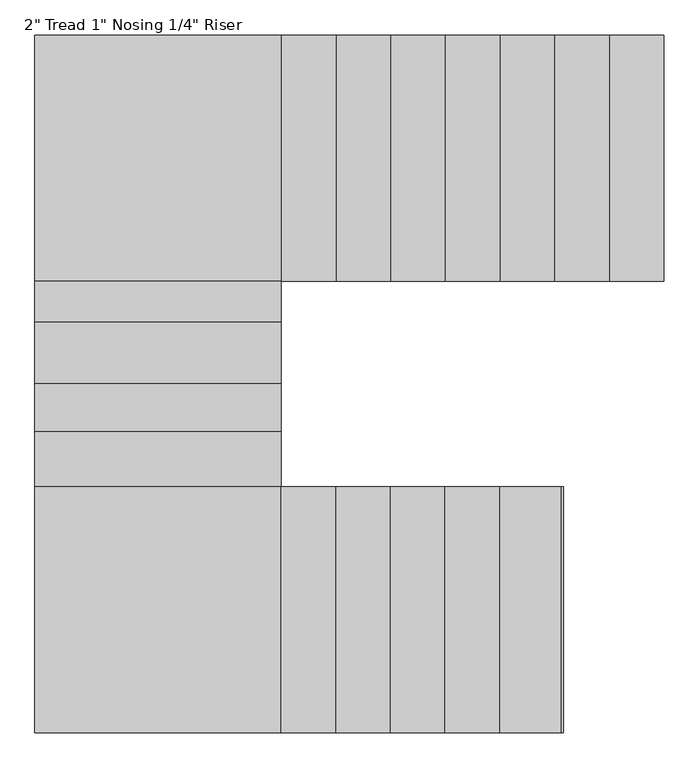
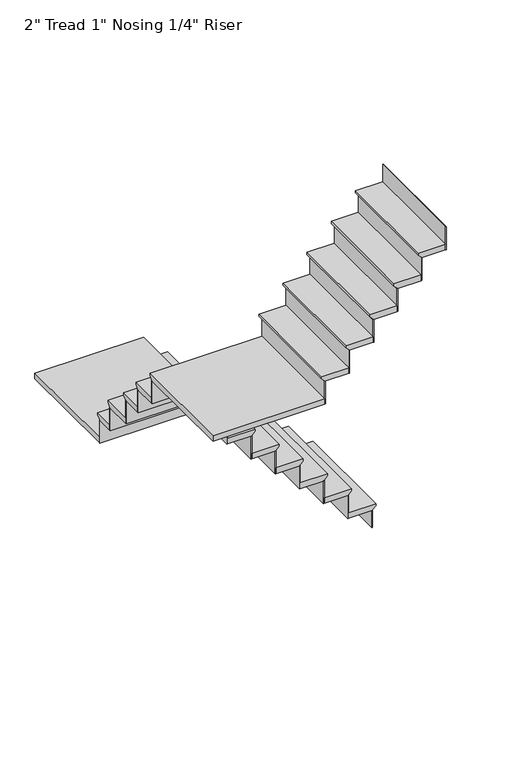
"""IFC4 building model written with IfcOpenShell, lengths in millimetres: stair flight geometry."""

from ifc_helpers import new_model, si_unit, origin, place, context, project, spatial, faceted_brep, source, transform, mapped, element, save


def stair_flight_8f890541(model_context):
    return source(origin(), model_context, "Body", "Brep", [
        faceted_brep([(-3603.1340247, 922.0319954, 184.15), (-3603.1340247, 922.0319954, 203.2), (-3603.1340247, 7.6319954, 203.2), (-3603.1340247, 7.6319954, 184.15), (-3628.5340247, 922.0319954, 158.75), (-3628.5340247, 7.6319954, 158.75), (-3831.7340247, 922.0319954, 203.2), (-3831.7340247, 7.6319954, 203.2), (-3628.5340247, 7.6319954, 152.4), (-3831.7340247, 7.6319954, 152.4), (-3831.7340247, 922.0319954, 152.4), (-3628.5340247, 922.0319954, 152.4)], [[[0, 1, 2, 3]], [[4, 0, 3, 5]], [[2, 1, 6, 7]], [[8, 9, 10, 11]], [[2, 7, 9, 8, 5, 3]], [[8, 11, 4, 5]], [[6, 1, 0, 4, 11, 10]], [[7, 6, 10, 9]]]),
        faceted_brep([(-3628.5340247, 922.0319954, 152.4), (-3628.5340247, 922.0319954, 0.0), (-3634.8840247, 922.0319954, 0.0), (-3634.8840247, 922.0319954, 152.4), (-3628.5340247, 7.6319954, 152.4), (-3634.8840247, 7.6319954, 152.4), (-3634.8840247, 7.6319954, 0.0), (-3628.5340247, 7.6319954, 0.0)], [[[0, 1, 2, 3]], [[4, 5, 6, 7]], [[1, 0, 4, 7]], [[2, 1, 7, 6]], [[3, 2, 6, 5]], [[0, 3, 5, 4]]]),
        faceted_brep([(-3831.7340247, 922.0319954, 355.6), (-3831.7340247, 922.0319954, 152.4), (-3838.0840247, 922.0319954, 152.4), (-3838.0840247, 922.0319954, 355.6), (-3831.7340247, 7.6319954, 355.6), (-3838.0840247, 7.6319954, 355.6), (-3838.0840247, 7.6319954, 152.4), (-3831.7340247, 7.6319954, 152.4)], [[[0, 1, 2, 3]], [[4, 5, 6, 7]], [[1, 0, 4, 7]], [[2, 1, 7, 6]], [[3, 2, 6, 5]], [[0, 3, 5, 4]]]),
        faceted_brep([(-3806.3340247, 7.6319954, 406.4), (-3806.3340247, 922.0319954, 406.4), (-4034.9340247, 922.0319954, 406.4), (-4034.9340247, 7.6319954, 406.4), (-3831.7340247, 7.6319954, 355.6), (-4034.9340247, 7.6319954, 355.6), (-4034.9340247, 922.0319954, 355.6), (-3831.7340247, 922.0319954, 355.6), (-3831.7340247, 7.6319954, 361.95), (-3806.3340247, 7.6319954, 387.35), (-3831.7340247, 922.0319954, 361.95), (-3806.3340247, 922.0319954, 387.35)], [[[0, 1, 2, 3]], [[4, 5, 6, 7]], [[0, 3, 5, 4, 8, 9]], [[4, 7, 10, 8]], [[2, 1, 11, 10, 7, 6]], [[3, 2, 6, 5]], [[11, 1, 0, 9]], [[10, 11, 9, 8]]]),
        faceted_brep([(-4034.9340247, 922.0319954, 558.8), (-4034.9340247, 922.0319954, 355.6), (-4041.2840247, 922.0319954, 355.6), (-4041.2840247, 922.0319954, 558.8), (-4034.9340247, 7.6319954, 558.8), (-4041.2840247, 7.6319954, 558.8), (-4041.2840247, 7.6319954, 355.6), (-4034.9340247, 7.6319954, 355.6)], [[[0, 1, 2, 3]], [[4, 5, 6, 7]], [[1, 0, 4, 7]], [[2, 1, 7, 6]], [[3, 2, 6, 5]], [[0, 3, 5, 4]]]),
        faceted_brep([(-4009.5340247, 7.6319954, 609.6), (-4009.5340247, 922.0319954, 609.6), (-4238.1340247, 922.0319954, 609.6), (-4238.1340247, 7.6319954, 609.6), (-4034.9340247, 7.6319954, 558.8), (-4238.1340247, 7.6319954, 558.8), (-4238.1340247, 922.0319954, 558.8), (-4034.9340247, 922.0319954, 558.8), (-4034.9340247, 7.6319954, 565.15), (-4009.5340247, 7.6319954, 590.55), (-4034.9340247, 922.0319954, 565.15), (-4009.5340247, 922.0319954, 590.55)], [[[0, 1, 2, 3]], [[4, 5, 6, 7]], [[0, 3, 5, 4, 8, 9]], [[4, 7, 10, 8]], [[2, 1, 11, 10, 7, 6]], [[3, 2, 6, 5]], [[11, 1, 0, 9]], [[10, 11, 9, 8]]]),
        faceted_brep([(-4238.1340247, 922.0319954, 762.0), (-4238.1340247, 922.0319954, 558.8), (-4244.4840247, 922.0319954, 558.8), (-4244.4840247, 922.0319954, 762.0), (-4238.1340247, 7.6319954, 762.0), (-4244.4840247, 7.6319954, 762.0), (-4244.4840247, 7.6319954, 558.8), (-4238.1340247, 7.6319954, 558.8)], [[[0, 1, 2, 3]], [[4, 5, 6, 7]], [[1, 0, 4, 7]], [[2, 1, 7, 6]], [[3, 2, 6, 5]], [[0, 3, 5, 4]]]),
        faceted_brep([(-4212.7340247, 7.6319954, 812.8), (-4212.7340247, 922.0319954, 812.8), (-4441.3340247, 922.0319954, 812.8), (-4441.3340247, 7.6319954, 812.8), (-4238.1340247, 7.6319954, 762.0), (-4441.3340247, 7.6319954, 762.0), (-4441.3340247, 922.0319954, 762.0), (-4238.1340247, 922.0319954, 762.0), (-4238.1340247, 7.6319954, 768.35), (-4212.7340247, 7.6319954, 793.75), (-4238.1340247, 922.0319954, 768.35), (-4212.7340247, 922.0319954, 793.75)], [[[0, 1, 2, 3]], [[4, 5, 6, 7]], [[0, 3, 5, 4, 8, 9]], [[4, 7, 10, 8]], [[2, 1, 11, 10, 7, 6]], [[3, 2, 6, 5]], [[11, 1, 0, 9]], [[10, 11, 9, 8]]]),
        faceted_brep([(-4441.3340247, 922.0319954, 965.2), (-4441.3340247, 922.0319954, 762.0), (-4447.6840247, 922.0319954, 762.0), (-4447.6840247, 922.0319954, 965.2), (-4441.3340247, 7.6319954, 965.2), (-4447.6840247, 7.6319954, 965.2), (-4447.6840247, 7.6319954, 762.0), (-4441.3340247, 7.6319954, 762.0)], [[[0, 1, 2, 3]], [[4, 5, 6, 7]], [[1, 0, 4, 7]], [[2, 1, 7, 6]], [[3, 2, 6, 5]], [[0, 3, 5, 4]]]),
        faceted_brep([(-4415.9340247, 7.6319954, 1016.0), (-4415.9340247, 922.0319954, 1016.0), (-4644.5340247, 922.0319954, 1016.0), (-4644.5340247, 7.6319954, 1016.0), (-4441.3340247, 7.6319954, 965.2), (-4644.5340247, 7.6319954, 965.2), (-4644.5340247, 922.0319954, 965.2), (-4441.3340247, 922.0319954, 965.2), (-4441.3340247, 7.6319954, 971.55), (-4415.9340247, 7.6319954, 996.95), (-4441.3340247, 922.0319954, 971.55), (-4415.9340247, 922.0319954, 996.95)], [[[0, 1, 2, 3]], [[4, 5, 6, 7]], [[0, 3, 5, 4, 8, 9]], [[4, 7, 10, 8]], [[2, 1, 11, 10, 7, 6]], [[3, 2, 6, 5]], [[11, 1, 0, 9]], [[10, 11, 9, 8]]]),
        faceted_brep([(-4644.5340247, 922.0319954, 1168.4), (-4644.5340247, 922.0319954, 965.2), (-4650.8840247, 922.0319954, 965.2), (-4650.8840247, 922.0319954, 1168.4), (-4644.5340247, 7.6319954, 1168.4), (-4650.8840247, 7.6319954, 1168.4), (-4650.8840247, 7.6319954, 965.2), (-4644.5340247, 7.6319954, 965.2)], [[[0, 1, 2, 3]], [[4, 5, 6, 7]], [[1, 0, 4, 7]], [[2, 1, 7, 6]], [[3, 2, 6, 5]], [[0, 3, 5, 4]]]),
        faceted_brep([(-4619.1340247, 7.6319954, 1219.2), (-4619.1340247, 922.0319954, 1219.2), (-4847.7340247, 922.0319954, 1219.2), (-4847.7340247, 7.6319954, 1219.2), (-4644.5340247, 7.6319954, 1168.4), (-4847.7340247, 7.6319954, 1168.4), (-4847.7340247, 922.0319954, 1168.4), (-4644.5340247, 922.0319954, 1168.4), (-4644.5340247, 7.6319954, 1174.75), (-4619.1340247, 7.6319954, 1200.15), (-4644.5340247, 922.0319954, 1174.75), (-4619.1340247, 922.0319954, 1200.15)], [[[0, 1, 2, 3]], [[4, 5, 6, 7]], [[0, 3, 5, 4, 8, 9]], [[4, 7, 10, 8]], [[2, 1, 11, 10, 7, 6]], [[3, 2, 6, 5]], [[11, 1, 0, 9]], [[10, 11, 9, 8]]]),
        faceted_brep([(-4847.7340247, 922.0319954, 1371.6), (-4847.7340247, 922.0319954, 1168.4), (-4854.0840247, 922.0319954, 1168.4), (-4854.0840247, 922.0319954, 1371.6), (-4847.7340247, 7.6319954, 1371.6), (-4854.0840247, 7.6319954, 1371.6), (-4854.0840247, 7.6319954, 1168.4), (-4847.7340247, 7.6319954, 1168.4)], [[[0, 1, 2, 3]], [[4, 5, 6, 7]], [[1, 0, 4, 7]], [[2, 1, 7, 6]], [[3, 2, 6, 5]], [[0, 3, 5, 4]]]),
        faceted_brep([(-4822.3340247, 7.6319954, 1422.4), (-4822.3340247, 922.0319954, 1422.4), (-5050.9340247, 922.0319954, 1422.4), (-5050.9340247, 7.6319954, 1422.4), (-4847.7340247, 7.6319954, 1371.6), (-5050.9340247, 7.6319954, 1371.6), (-5050.9340247, 922.0319954, 1371.6), (-4847.7340247, 922.0319954, 1371.6), (-4847.7340247, 7.6319954, 1377.95), (-4822.3340247, 7.6319954, 1403.35), (-4847.7340247, 922.0319954, 1377.95), (-4822.3340247, 922.0319954, 1403.35)], [[[0, 1, 2, 3]], [[4, 5, 6, 7]], [[0, 3, 5, 4, 8, 9]], [[4, 7, 10, 8]], [[2, 1, 11, 10, 7, 6]], [[3, 2, 6, 5]], [[11, 1, 0, 9]], [[10, 11, 9, 8]]]),
        faceted_brep([(-5050.9340247, 922.0319954, 1574.8), (-5050.9340247, 922.0319954, 1371.6), (-5057.2840247, 922.0319954, 1371.6), (-5057.2840247, 922.0319954, 1574.8), (-5050.9340247, 7.6319954, 1574.8), (-5057.2840247, 7.6319954, 1574.8), (-5057.2840247, 7.6319954, 1371.6), (-5050.9340247, 7.6319954, 1371.6)], [[[0, 1, 2, 3]], [[4, 5, 6, 7]], [[1, 0, 4, 7]], [[2, 1, 7, 6]], [[3, 2, 6, 5]], [[0, 3, 5, 4]]]),
        faceted_brep([(-5939.9340247, 922.0319954, 1625.6), (-5939.9340247, -17.7680046, 1625.6), (-5025.5340247, -17.7680046, 1625.6), (-5025.5340247, 922.0319954, 1625.6), (-5025.5340247, 7.6319954, 1574.8), (-5025.5340247, -17.7680046, 1574.8), (-5939.9340247, -17.7680046, 1574.8), (-5939.9340247, 922.0319954, 1574.8), (-5050.9340247, 922.0319954, 1574.8), (-5050.9340247, 7.6319954, 1574.8), (-5025.5340247, 7.6319954, 1606.55), (-5025.5340247, 922.0319954, 1606.55), (-5050.9340247, 7.6319954, 1581.15), (-5050.9340247, 922.0319954, 1581.15)], [[[0, 1, 2, 3]], [[4, 5, 6, 7, 8, 9]], [[3, 2, 5, 4, 10, 11]], [[4, 9, 12, 10]], [[9, 8, 13, 12]], [[0, 3, 11, 13, 8, 7]], [[1, 0, 7, 6]], [[2, 1, 6, 5]], [[13, 11, 10, 12]]]),
        faceted_brep([(-5939.9340247, -17.7680046, 1778.0), (-5939.9340247, -17.7680046, 1574.8), (-5939.9340247, -24.1180046, 1574.8), (-5939.9340247, -24.1180046, 1778.0), (-5025.5340247, -17.7680046, 1778.0), (-5025.5340247, -24.1180046, 1778.0), (-5025.5340247, -24.1180046, 1574.8), (-5025.5340247, -17.7680046, 1574.8)], [[[0, 1, 2, 3]], [[4, 5, 6, 7]], [[1, 0, 4, 7]], [[2, 1, 7, 6]], [[3, 2, 6, 5]], [[0, 3, 5, 4]]]),
        faceted_brep([(-5025.5340247, 7.6319954, 1828.8), (-5939.9340247, 7.6319954, 1828.8), (-5939.9340247, -170.1680046, 1828.8), (-5025.5340247, -170.1680046, 1828.8), (-5025.5340247, -17.7680046, 1778.0), (-5025.5340247, -170.1680046, 1778.0), (-5939.9340247, -170.1680046, 1778.0), (-5939.9340247, -17.7680046, 1778.0), (-5025.5340247, -17.7680046, 1784.35), (-5025.5340247, 7.6319954, 1809.75), (-5939.9340247, -17.7680046, 1784.35), (-5939.9340247, 7.6319954, 1809.75)], [[[0, 1, 2, 3]], [[4, 5, 6, 7]], [[0, 3, 5, 4, 8, 9]], [[4, 7, 10, 8]], [[2, 1, 11, 10, 7, 6]], [[3, 2, 6, 5]], [[11, 1, 0, 9]], [[10, 11, 9, 8]]]),
        faceted_brep([(-5939.9340247, -170.1680046, 1981.2), (-5939.9340247, -170.1680046, 1778.0), (-5939.9340247, -176.5180046, 1778.0), (-5939.9340247, -176.5180046, 1981.2), (-5025.5340247, -170.1680046, 1981.2), (-5025.5340247, -176.5180046, 1981.2), (-5025.5340247, -176.5180046, 1778.0), (-5025.5340247, -170.1680046, 1778.0)], [[[0, 1, 2, 3]], [[4, 5, 6, 7]], [[1, 0, 4, 7]], [[2, 1, 7, 6]], [[3, 2, 6, 5]], [[0, 3, 5, 4]]]),
        faceted_brep([(-5025.5340247, -144.7680046, 2032.0), (-5939.9340247, -144.7680046, 2032.0), (-5939.9340247, -398.7680046, 2032.0), (-5025.5340247, -398.7680046, 2032.0), (-5025.5340247, -170.1680046, 1981.2), (-5025.5340247, -398.7680046, 1981.2), (-5939.9340247, -398.7680046, 1981.2), (-5939.9340247, -170.1680046, 1981.2), (-5025.5340247, -170.1680046, 1987.55), (-5025.5340247, -144.7680046, 2012.95), (-5939.9340247, -170.1680046, 1987.55), (-5939.9340247, -144.7680046, 2012.95)], [[[0, 1, 2, 3]], [[4, 5, 6, 7]], [[0, 3, 5, 4, 8, 9]], [[4, 7, 10, 8]], [[2, 1, 11, 10, 7, 6]], [[3, 2, 6, 5]], [[11, 1, 0, 9]], [[10, 11, 9, 8]]]),
        faceted_brep([(-5939.9340247, -398.7680046, 2184.4), (-5939.9340247, -398.7680046, 1981.2), (-5939.9340247, -405.1180046, 1981.2), (-5939.9340247, -405.1180046, 2184.4), (-5025.5340247, -398.7680046, 2184.4), (-5025.5340247, -405.1180046, 2184.4), (-5025.5340247, -405.1180046, 1981.2), (-5025.5340247, -398.7680046, 1981.2)], [[[0, 1, 2, 3]], [[4, 5, 6, 7]], [[1, 0, 4, 7]], [[2, 1, 7, 6]], [[3, 2, 6, 5]], [[0, 3, 5, 4]]]),
        faceted_brep([(-5025.5340247, -373.3680046, 2235.2), (-5939.9340247, -373.3680046, 2235.2), (-5939.9340247, -576.5680046, 2235.2), (-5025.5340247, -576.5680046, 2235.2), (-5025.5340247, -398.7680046, 2184.4), (-5025.5340247, -576.5680046, 2184.4), (-5939.9340247, -576.5680046, 2184.4), (-5939.9340247, -398.7680046, 2184.4), (-5025.5340247, -398.7680046, 2190.75), (-5025.5340247, -373.3680046, 2216.15), (-5939.9340247, -398.7680046, 2190.75), (-5939.9340247, -373.3680046, 2216.15)], [[[0, 1, 2, 3]], [[4, 5, 6, 7]], [[0, 3, 5, 4, 8, 9]], [[4, 7, 10, 8]], [[2, 1, 11, 10, 7, 6]], [[3, 2, 6, 5]], [[11, 1, 0, 9]], [[10, 11, 9, 8]]]),
        faceted_brep([(-5939.9340247, -576.5680046, 2387.6), (-5939.9340247, -576.5680046, 2184.4), (-5939.9340247, -582.9180046, 2184.4), (-5939.9340247, -582.9180046, 2387.6), (-5025.5340247, -576.5680046, 2387.6), (-5025.5340247, -582.9180046, 2387.6), (-5025.5340247, -582.9180046, 2184.4), (-5025.5340247, -576.5680046, 2184.4)], [[[0, 1, 2, 3]], [[4, 5, 6, 7]], [[1, 0, 4, 7]], [[2, 1, 7, 6]], [[3, 2, 6, 5]], [[0, 3, 5, 4]]]),
        faceted_brep([(-5025.5340247, -551.1680046, 2438.4), (-5939.9340247, -551.1680046, 2438.4), (-5939.9340247, -779.7680046, 2438.4), (-5025.5340247, -779.7680046, 2438.4), (-5025.5340247, -576.5680046, 2387.6), (-5025.5340247, -779.7680046, 2387.6), (-5939.9340247, -779.7680046, 2387.6), (-5939.9340247, -576.5680046, 2387.6), (-5025.5340247, -576.5680046, 2393.95), (-5025.5340247, -551.1680046, 2419.35), (-5939.9340247, -576.5680046, 2393.95), (-5939.9340247, -551.1680046, 2419.35)], [[[0, 1, 2, 3]], [[4, 5, 6, 7]], [[0, 3, 5, 4, 8, 9]], [[4, 7, 10, 8]], [[2, 1, 11, 10, 7, 6]], [[3, 2, 6, 5]], [[11, 1, 0, 9]], [[10, 11, 9, 8]]]),
        faceted_brep([(-5939.9340247, -779.7680046, 2590.8), (-5939.9340247, -779.7680046, 2387.6), (-5939.9340247, -786.1180046, 2387.6), (-5939.9340247, -786.1180046, 2590.8), (-5025.5340247, -779.7680046, 2590.8), (-5025.5340247, -786.1180046, 2590.8), (-5025.5340247, -786.1180046, 2387.6), (-5025.5340247, -779.7680046, 2387.6)], [[[0, 1, 2, 3]], [[4, 5, 6, 7]], [[1, 0, 4, 7]], [[2, 1, 7, 6]], [[3, 2, 6, 5]], [[0, 3, 5, 4]]]),
        faceted_brep([(-5939.9340247, -1668.7680046, 2641.6), (-5000.1340247, -1668.7680046, 2641.6), (-5000.1340247, -754.3680046, 2641.6), (-5939.9340247, -754.3680046, 2641.6), (-5025.5340247, -754.3680046, 2590.8), (-5000.1340247, -754.3680046, 2590.8), (-5000.1340247, -1668.7680046, 2590.8), (-5939.9340247, -1668.7680046, 2590.8), (-5939.9340247, -779.7680046, 2590.8), (-5025.5340247, -779.7680046, 2590.8), (-5025.5340247, -754.3680046, 2622.55), (-5939.9340247, -754.3680046, 2622.55), (-5025.5340247, -779.7680046, 2597.15), (-5939.9340247, -779.7680046, 2597.15)], [[[0, 1, 2, 3]], [[4, 5, 6, 7, 8, 9]], [[3, 2, 5, 4, 10, 11]], [[4, 9, 12, 10]], [[9, 8, 13, 12]], [[0, 3, 11, 13, 8, 7]], [[1, 0, 7, 6]], [[2, 1, 6, 5]], [[13, 11, 10, 12]]]),
        faceted_brep([(-5000.1340247, -1668.7680046, 2794.0), (-5000.1340247, -1668.7680046, 2590.8), (-4993.7840247, -1668.7680046, 2590.8), (-4993.7840247, -1668.7680046, 2794.0), (-5000.1340247, -754.3680046, 2794.0), (-4993.7840247, -754.3680046, 2794.0), (-4993.7840247, -754.3680046, 2590.8), (-5000.1340247, -754.3680046, 2590.8)], [[[0, 1, 2, 3]], [[4, 5, 6, 7]], [[1, 0, 4, 7]], [[2, 1, 7, 6]], [[3, 2, 6, 5]], [[0, 3, 5, 4]]]),
        faceted_brep([(-5025.5340247, -754.3680046, 2844.8), (-5025.5340247, -1668.7680046, 2844.8), (-4796.9340247, -1668.7680046, 2844.8), (-4796.9340247, -754.3680046, 2844.8), (-5000.1340247, -754.3680046, 2794.0), (-4796.9340247, -754.3680046, 2794.0), (-4796.9340247, -1668.7680046, 2794.0), (-5000.1340247, -1668.7680046, 2794.0), (-5000.1340247, -754.3680046, 2800.35), (-5025.5340247, -754.3680046, 2825.75), (-5000.1340247, -1668.7680046, 2800.35), (-5025.5340247, -1668.7680046, 2825.75)], [[[0, 1, 2, 3]], [[4, 5, 6, 7]], [[0, 3, 5, 4, 8, 9]], [[4, 7, 10, 8]], [[2, 1, 11, 10, 7, 6]], [[3, 2, 6, 5]], [[11, 1, 0, 9]], [[10, 11, 9, 8]]]),
        faceted_brep([(-4796.9340247, -1668.7680046, 2997.2), (-4796.9340247, -1668.7680046, 2794.0), (-4790.5840247, -1668.7680046, 2794.0), (-4790.5840247, -1668.7680046, 2997.2), (-4796.9340247, -754.3680046, 2997.2), (-4790.5840247, -754.3680046, 2997.2), (-4790.5840247, -754.3680046, 2794.0), (-4796.9340247, -754.3680046, 2794.0)], [[[0, 1, 2, 3]], [[4, 5, 6, 7]], [[1, 0, 4, 7]], [[2, 1, 7, 6]], [[3, 2, 6, 5]], [[0, 3, 5, 4]]]),
        faceted_brep([(-4822.3340247, -754.3680046, 3048.0), (-4822.3340247, -1668.7680046, 3048.0), (-4593.7340247, -1668.7680046, 3048.0), (-4593.7340247, -754.3680046, 3048.0), (-4796.9340247, -754.3680046, 2997.2), (-4593.7340247, -754.3680046, 2997.2), (-4593.7340247, -1668.7680046, 2997.2), (-4796.9340247, -1668.7680046, 2997.2), (-4796.9340247, -754.3680046, 3003.55), (-4822.3340247, -754.3680046, 3028.95), (-4796.9340247, -1668.7680046, 3003.55), (-4822.3340247, -1668.7680046, 3028.95)], [[[0, 1, 2, 3]], [[4, 5, 6, 7]], [[0, 3, 5, 4, 8, 9]], [[4, 7, 10, 8]], [[2, 1, 11, 10, 7, 6]], [[3, 2, 6, 5]], [[11, 1, 0, 9]], [[10, 11, 9, 8]]]),
        faceted_brep([(-4593.7340247, -1668.7680046, 3200.4), (-4593.7340247, -1668.7680046, 2997.2), (-4587.3840247, -1668.7680046, 2997.2), (-4587.3840247, -1668.7680046, 3200.4), (-4593.7340247, -754.3680046, 3200.4), (-4587.3840247, -754.3680046, 3200.4), (-4587.3840247, -754.3680046, 2997.2), (-4593.7340247, -754.3680046, 2997.2)], [[[0, 1, 2, 3]], [[4, 5, 6, 7]], [[1, 0, 4, 7]], [[2, 1, 7, 6]], [[3, 2, 6, 5]], [[0, 3, 5, 4]]]),
        faceted_brep([(-4619.1340247, -754.3680046, 3251.2), (-4619.1340247, -1668.7680046, 3251.2), (-4390.5340247, -1668.7680046, 3251.2), (-4390.5340247, -754.3680046, 3251.2), (-4593.7340247, -754.3680046, 3200.4), (-4390.5340247, -754.3680046, 3200.4), (-4390.5340247, -1668.7680046, 3200.4), (-4593.7340247, -1668.7680046, 3200.4), (-4593.7340247, -754.3680046, 3206.75), (-4619.1340247, -754.3680046, 3232.15), (-4593.7340247, -1668.7680046, 3206.75), (-4619.1340247, -1668.7680046, 3232.15)], [[[0, 1, 2, 3]], [[4, 5, 6, 7]], [[0, 3, 5, 4, 8, 9]], [[4, 7, 10, 8]], [[2, 1, 11, 10, 7, 6]], [[3, 2, 6, 5]], [[11, 1, 0, 9]], [[10, 11, 9, 8]]]),
        faceted_brep([(-4390.5340247, -1668.7680046, 3403.6), (-4390.5340247, -1668.7680046, 3200.4), (-4384.1840247, -1668.7680046, 3200.4), (-4384.1840247, -1668.7680046, 3403.6), (-4390.5340247, -754.3680046, 3403.6), (-4384.1840247, -754.3680046, 3403.6), (-4384.1840247, -754.3680046, 3200.4), (-4390.5340247, -754.3680046, 3200.4)], [[[0, 1, 2, 3]], [[4, 5, 6, 7]], [[1, 0, 4, 7]], [[2, 1, 7, 6]], [[3, 2, 6, 5]], [[0, 3, 5, 4]]]),
        faceted_brep([(-4415.9340247, -754.3680046, 3454.4), (-4415.9340247, -1668.7680046, 3454.4), (-4187.3340247, -1668.7680046, 3454.4), (-4187.3340247, -754.3680046, 3454.4), (-4390.5340247, -754.3680046, 3403.6), (-4187.3340247, -754.3680046, 3403.6), (-4187.3340247, -1668.7680046, 3403.6), (-4390.5340247, -1668.7680046, 3403.6), (-4390.5340247, -754.3680046, 3409.95), (-4415.9340247, -754.3680046, 3435.35), (-4390.5340247, -1668.7680046, 3409.95), (-4415.9340247, -1668.7680046, 3435.35)], [[[0, 1, 2, 3]], [[4, 5, 6, 7]], [[0, 3, 5, 4, 8, 9]], [[4, 7, 10, 8]], [[2, 1, 11, 10, 7, 6]], [[3, 2, 6, 5]], [[11, 1, 0, 9]], [[10, 11, 9, 8]]]),
        faceted_brep([(-4187.3340247, -1668.7680046, 3606.8), (-4187.3340247, -1668.7680046, 3403.6), (-4180.9840247, -1668.7680046, 3403.6), (-4180.9840247, -1668.7680046, 3606.8), (-4187.3340247, -754.3680046, 3606.8), (-4180.9840247, -754.3680046, 3606.8), (-4180.9840247, -754.3680046, 3403.6), (-4187.3340247, -754.3680046, 3403.6)], [[[0, 1, 2, 3]], [[4, 5, 6, 7]], [[1, 0, 4, 7]], [[2, 1, 7, 6]], [[3, 2, 6, 5]], [[0, 3, 5, 4]]]),
        faceted_brep([(-3984.1340247, -1668.7680046, 3810.0), (-3984.1340247, -1668.7680046, 3606.8), (-3977.7840247, -1668.7680046, 3606.8), (-3977.7840247, -1668.7680046, 3810.0), (-3984.1340247, -754.3680046, 3810.0), (-3977.7840247, -754.3680046, 3810.0), (-3977.7840247, -754.3680046, 3606.8), (-3984.1340247, -754.3680046, 3606.8)], [[[0, 1, 2, 3]], [[4, 5, 6, 7]], [[1, 0, 4, 7]], [[2, 1, 7, 6]], [[3, 2, 6, 5]], [[0, 3, 5, 4]]]),
        faceted_brep([(-4212.7340247, -754.3680046, 3657.6), (-4212.7340247, -1668.7680046, 3657.6), (-3984.1340247, -1668.7680046, 3657.6), (-3984.1340247, -754.3680046, 3657.6), (-4187.3340247, -754.3680046, 3606.8), (-3984.1340247, -754.3680046, 3606.8), (-3984.1340247, -1668.7680046, 3606.8), (-4187.3340247, -1668.7680046, 3606.8), (-4187.3340247, -754.3680046, 3613.15), (-4212.7340247, -754.3680046, 3638.55), (-4187.3340247, -1668.7680046, 3613.15), (-4212.7340247, -1668.7680046, 3638.55)], [[[0, 1, 2, 3]], [[4, 5, 6, 7]], [[0, 3, 5, 4, 8, 9]], [[4, 7, 10, 8]], [[2, 1, 11, 10, 7, 6]], [[3, 2, 6, 5]], [[11, 1, 0, 9]], [[10, 11, 9, 8]]]),
    ])


if __name__ == "__main__":
    model = new_model("IFC4")
    model_context = context("Model", 3, world=origin())
    ifc_project = project(units=[si_unit("LENGTHUNIT", "METRE", prefix="MILLI")], contexts=[model_context])
    site = spatial("IfcSite", under=ifc_project)
    building = spatial("IfcBuilding", under=site)
    placement = place(None, origin())
    stair_flight_shape = stair_flight_8f890541(model_context)
    element("IfcStairFlight", 1, ObjectType="2\" Tread 1\" Nosing 1/4\" Riser", at=placement, inside=building, context=model_context, shape_type="MappedRepresentation", body=[
        mapped(stair_flight_shape, transform((0.0, 0.0, 0.0), x_axis=(1.0, 0.0, 0.0), y_axis=(0.0, 1.0, 0.0), z_axis=(0.0, 0.0, 1.0))),
    ])
    save(model, "model.ifc")
